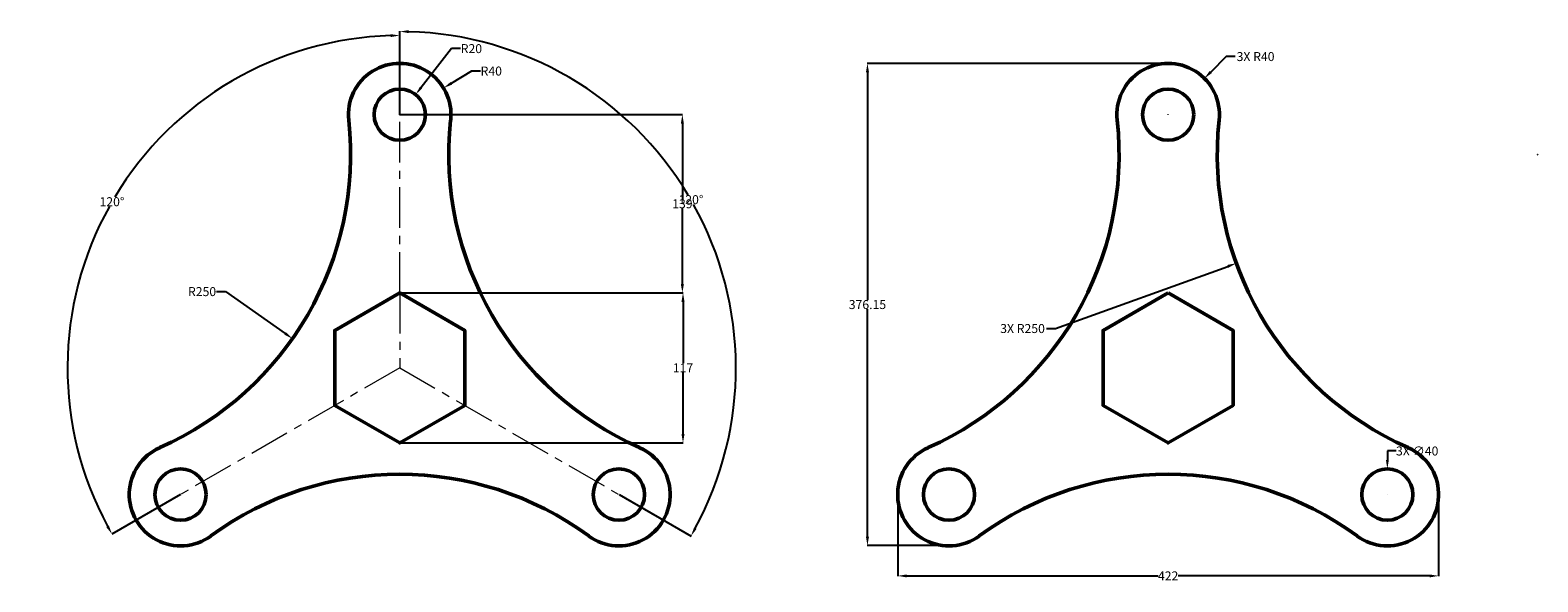
# Model space of a CAD drawing. Units: millimetres. Extents: x 13 to 1189, y 87 to 517.
import ezdxf

# ---------------------------------------------------------------- set-up
doc = ezdxf.new("R2010")
doc.units = ezdxf.units.MM
doc.header["$MEASUREMENT"] = 0
doc.linetypes.add('CENTER', pattern=[50.8, 31.75, -6.35, 6.35, -6.35])
for name, color, linetype, lineweight in [('M-CNTR', 7, 'CENTER', 18), ('M-DIMS', 3, 'Continuous', 25), ('M-OUTL', 7, 'Continuous', 50)]:
    doc.layers.add(name, color=color, linetype=linetype, lineweight=lineweight)
doc.styles.get("Standard").update_dxf_attribs({"font": 'arial.ttf'})
doc.dimstyles.get("Standard").update_dxf_attribs({"dimtxt": 7, "dimasz": 7, "dimexe": 0.18, "dimexo": 0.0625, "dimgap": 0.09, "dimtad": 0, "dimtih": 1, "dimtoh": 1, "dimdec": 1, "dimdsep": 46, "dimtxsty": 'Standard', "dimcen": 0.09, "dimadec": 0, "dimazin": 0, "dimtfac": 1, "dimtdec": 1, "dimtofl": 0, "dimtmove": 0, "dimatfit": 3, "dimfxl": 1, "dimtolj": 1, "dimtzin": 0, "dimarcsym": 0})

# ---------------------------------------------------------------- blocks, each defined once
blk = doc.blocks.new('*D1')
at = {"layer": 'Defpoints', "color": 0, "transparency": 16777216}
for p in [(301, 312.5), (522, 312.5), (301, 195.5)]:
    blk.add_point(p, dxfattribs=at)
at = {"layer": 'M-DIMS', "color": 0, "lineweight": -2, "transparency": 16777216}
for p, q in [((301.1, 312.5), (522.2, 312.5)), ((522, 305.5), (522, 257.6)), ((522, 202.5), (522, 250.4)), ((301.1, 195.5), (522.2, 195.5))]:
    blk.add_line(p, q, dxfattribs=at)
at = {"layer": 'M-DIMS', "color": 0, "transparency": 16777216}
for points in [[(520.8, 305.5), (523.2, 305.5), (522, 312.5)], [(520.8, 202.5), (523.2, 202.5), (522, 195.5)]]:
    blk.add_solid(points, dxfattribs=at)
at = {"layer": 'M-DIMS', "color": 0, "transparency": 16777216, "insert": (522, 254), "char_height": 7, "attachment_point": 5}
blk.add_mtext('\\A1;117', dxfattribs=at)
blk = doc.blocks.new('*D2')
at = {"layer": 'Defpoints', "color": 0, "transparency": 16777216}
for p in [(301, 451.5), (521.5, 451.5), (301, 312.5)]:
    blk.add_point(p, dxfattribs=at)
at = {"layer": 'M-DIMS', "color": 0, "lineweight": -2, "transparency": 16777216}
for p, q in [((301.1, 451.5), (521.7, 451.5)), ((521.5, 444.5), (521.5, 385.7)), ((521.5, 319.5), (521.5, 378.3)), ((301.1, 312.5), (521.7, 312.5))]:
    blk.add_line(p, q, dxfattribs=at)
at = {"layer": 'M-DIMS', "color": 0, "transparency": 16777216}
for points in [[(520.3, 444.5), (522.7, 444.5), (521.5, 451.5)], [(520.3, 319.5), (522.7, 319.5), (521.5, 312.5)]]:
    blk.add_solid(points, dxfattribs=at)
at = {"layer": 'M-DIMS', "color": 0, "transparency": 16777216, "insert": (521.5, 382), "char_height": 7, "attachment_point": 5}
blk.add_mtext('\\A1;139', dxfattribs=at)
blk = doc.blocks.new('*D3')
at = {"layer": 'Defpoints', "color": 0, "transparency": 16777216}
for p in [(313.4, 467.2), (301, 451.5)]:
    blk.add_point(p, dxfattribs=at)
at = {"layer": 'M-DIMS', "color": 0, "lineweight": -2, "transparency": 16777216}
for p, q in [((341.5, 503), (317.7, 472.7)), ((348.5, 503), (341.5, 503)), ((300.9, 451.5), (301.1, 451.5)), ((301, 451.4), (301, 451.6))]:
    blk.add_line(p, q, dxfattribs=at)
at = {"layer": 'M-DIMS', "color": 0, "transparency": 16777216}
blk.add_solid([(316.8, 473.4), (318.6, 472), (313.4, 467.2)], dxfattribs=at)
at = {"layer": 'M-DIMS', "color": 0, "transparency": 16777216, "insert": (356.9, 503), "char_height": 7, "attachment_point": 5}
blk.add_mtext('\\A1;R20', dxfattribs=at)
blk = doc.blocks.new('*D4')
at = {"layer": 'Defpoints', "color": 0, "transparency": 16777216}
for p in [(335.2, 472.3), (301, 451.5)]:
    blk.add_point(p, dxfattribs=at)
at = {"layer": 'M-DIMS', "color": 0, "lineweight": -2, "transparency": 16777216}
for p, q in [((357, 485.5), (341.2, 475.9)), ((364, 485.5), (357, 485.5)), ((300.9, 451.5), (301.1, 451.5)), ((301, 451.4), (301, 451.6))]:
    blk.add_line(p, q, dxfattribs=at)
at = {"layer": 'M-DIMS', "color": 0, "transparency": 16777216}
blk.add_solid([(340.6, 476.9), (341.8, 474.9), (335.2, 472.3)], dxfattribs=at)
at = {"layer": 'M-DIMS', "color": 0, "transparency": 16777216, "insert": (372.4, 485.5), "char_height": 7, "attachment_point": 5}
blk.add_mtext('\\A1;R40', dxfattribs=at)
blk = doc.blocks.new('*D5')
at = {"layer": 'Defpoints', "color": 0, "transparency": 16777216}
for p in [(12.7, 420.5), (217.3, 276.8)]:
    blk.add_point(p, dxfattribs=at)
at = {"layer": 'M-DIMS', "color": 0, "lineweight": -2, "transparency": 16777216}
for p, q in [((158, 313.5), (165, 313.5)), ((165, 313.5), (211.5, 280.8))]:
    blk.add_line(p, q, dxfattribs=at)
at = {"layer": 'M-DIMS', "color": 0, "transparency": 16777216}
blk.add_solid([(212.2, 281.8), (210.9, 279.9), (217.3, 276.8)], dxfattribs=at)
at = {"layer": 'M-DIMS', "color": 0, "transparency": 16777216, "insert": (146.8, 313.5), "char_height": 7, "attachment_point": 5}
blk.add_mtext('\\A1;R250', dxfattribs=at)
blk = doc.blocks.new('*D6')
at = {"layer": 'Defpoints', "color": 0, "transparency": 16777216}
for p in [(134.4, 452.6), (301, 451.5), (301, 312.5), (301, 254), (130, 155.2)]:
    blk.add_point(p, dxfattribs=at)
at = {"layer": 'M-DIMS', "color": 0, "lineweight": -2, "transparency": 16777216}
for p, q in [((301, 451.6), (301, 513.4)), ((129.9, 155.2), (76.3, 124.3))]:
    blk.add_line(p, q, dxfattribs=at)
for start, end in [(91.5471, 149.0605), (150.9307, 208.4529)]:
    blk.add_arc((301, 254), 259.2, start, end, dxfattribs=at)
at = {"layer": 'M-DIMS', "color": 0, "transparency": 16777216}
for points in [[(294, 514.3), (294, 512), (301, 513.2)], [(74.1, 131.1), (72, 129.9), (76.5, 124.4)]]:
    blk.add_solid(points, dxfattribs=at)
at = {"layer": 'M-DIMS', "color": 0, "transparency": 16777216, "insert": (76.5, 383.6), "char_height": 7, "attachment_point": 5}
blk.add_mtext('\\A1;120°', dxfattribs=at)
blk = doc.blocks.new('*D7')
at = {"layer": 'Defpoints', "color": 0, "transparency": 16777216}
for p in [(301, 451.5), (301, 312.5), (559.3, 299.6), (301, 254), (472, 155.2)]:
    blk.add_point(p, dxfattribs=at)
at = {"layer": 'M-DIMS', "color": 0, "lineweight": -2, "transparency": 16777216}
for p, q in [((301, 451.6), (301, 516.5)), ((472.1, 155.2), (528.3, 122.8))]:
    blk.add_line(p, q, dxfattribs=at)
for start, end in [(30.9285, 88.471), (331.529, 29.0801)]:
    blk.add_arc((301, 254), 262.3, start, end, dxfattribs=at)
at = {"layer": 'M-DIMS', "color": 0, "transparency": 16777216}
for points in [[(308, 515.1), (308, 517.4), (301, 516.3)], [(532.6, 128.4), (530.6, 129.5), (528.2, 122.8)]]:
    blk.add_solid(points, dxfattribs=at)
at = {"layer": 'M-DIMS', "color": 0, "transparency": 16777216, "insert": (528.2, 385.2), "char_height": 7, "attachment_point": 5}
blk.add_mtext('\\A1;120°', dxfattribs=at)
blk = doc.blocks.new('PLATE-3ARM-HEX')
blk.add_lwpolyline([(0, 58.5), (-50.7, 29.2), (-50.7, -29.3), (0, -58.5), (50.7, -29.3), (50.7, 29.2)], close=True)
for centre in [(0, 197.5), (-171, -98.8), (171, -98.8)]:
    blk.add_circle(centre, 20)
for centre, radius, start, end in [((0, 197.5), 40, 353.8577, 186.1423), ((-288.3, 166.5), 250, 293.8577, 6.1423), ((288.3, 166.5), 250, 173.8577, 246.1423), ((-171, -98.8), 40, 113.8577, 306.1423), ((171, -98.8), 40, 233.8577, 66.1423), ((0, -332.9), 250, 53.8577, 126.1423)]:
    blk.add_arc(centre, radius, start, end)
blk = doc.blocks.new('*D9')
at = {"layer": 'Defpoints', "color": 0, "transparency": 16777216}
for p in [(689.5, 156.7), (1111.5, 156.7), (1111.5, 91.8)]:
    blk.add_point(p, dxfattribs=at)
at = {"layer": 'M-DIMS', "color": 0, "lineweight": -2, "transparency": 16777216}
for p, q in [((689.5, 156.6), (689.5, 91.6)), ((1111.5, 156.6), (1111.5, 91.6)), ((696.5, 91.8), (892.6, 91.8)), ((1104.5, 91.8), (908.4, 91.8))]:
    blk.add_line(p, q, dxfattribs=at)
at = {"layer": 'M-DIMS', "color": 0, "transparency": 16777216}
for points in [[(696.5, 92.9), (696.5, 90.6), (689.5, 91.8)], [(1104.5, 92.9), (1104.5, 90.6), (1111.5, 91.8)]]:
    blk.add_solid(points, dxfattribs=at)
at = {"layer": 'M-DIMS', "color": 0, "transparency": 16777216, "insert": (900.5, 91.8), "char_height": 7, "attachment_point": 5}
blk.add_mtext('\\A1;422', dxfattribs=at)
blk = doc.blocks.new('*D10')
at = {"layer": 'Defpoints', "color": 0, "transparency": 16777216}
for p in [(665.9, 491.5), (900.5, 491.5), (732.3, 115.4)]:
    blk.add_point(p, dxfattribs=at)
at = {"layer": 'M-DIMS', "color": 0, "lineweight": -2, "transparency": 16777216}
for p, q in [((900.4, 491.5), (665.7, 491.5)), ((665.9, 484.5), (665.9, 307.1)), ((665.9, 122.4), (665.9, 299.8)), ((732.3, 115.4), (665.7, 115.4))]:
    blk.add_line(p, q, dxfattribs=at)
at = {"layer": 'M-DIMS', "color": 0, "transparency": 16777216}
for points in [[(664.7, 484.5), (667.1, 484.5), (665.9, 491.5)], [(664.7, 122.4), (667.1, 122.4), (665.9, 115.4)]]:
    blk.add_solid(points, dxfattribs=at)
at = {"layer": 'M-DIMS', "color": 0, "transparency": 16777216, "insert": (665.9, 303.4), "char_height": 7, "attachment_point": 5}
blk.add_mtext('\\A1;376.15', dxfattribs=at)
blk = doc.blocks.new('*D11')
at = {"layer": 'Defpoints', "color": 0, "transparency": 16777216}
for p in [(1071.5, 175.3), (1071.5, 135.3)]:
    blk.add_point(p, dxfattribs=at)
at = {"layer": 'M-DIMS', "color": 0, "lineweight": -2, "transparency": 16777216}
for p, q in [((1078.5, 189.2), (1071.5, 189.2)), ((1071.5, 189.2), (1071.5, 182.3)), ((1071.5, 155.3), (1071.6, 155.3)), ((1071.5, 155.2), (1071.5, 155.3))]:
    blk.add_line(p, q, dxfattribs=at)
at = {"layer": 'M-DIMS', "color": 0, "transparency": 16777216}
blk.add_solid([(1070.4, 182.3), (1072.7, 182.3), (1071.5, 175.3)], dxfattribs=at)
at = {"layer": 'M-DIMS', "color": 0, "transparency": 16777216, "insert": (1094.8, 189.2), "char_height": 7, "attachment_point": 5}
blk.add_mtext('\\A1;3X ∅40', dxfattribs=at)
blk = doc.blocks.new('*D12')
at = {"layer": 'Defpoints', "color": 0, "transparency": 16777216}
for p in [(928.8, 479.8), (900.5, 451.5)]:
    blk.add_point(p, dxfattribs=at)
at = {"layer": 'M-DIMS', "color": 0, "lineweight": -2, "transparency": 16777216}
for p, q in [((945.8, 496.8), (933.7, 484.7)), ((952.8, 496.8), (945.8, 496.8)), ((900.4, 451.5), (900.6, 451.5)), ((900.5, 451.4), (900.5, 451.6))]:
    blk.add_line(p, q, dxfattribs=at)
at = {"layer": 'M-DIMS', "color": 0, "transparency": 16777216}
blk.add_solid([(932.9, 485.6), (934.6, 483.9), (928.8, 479.8)], dxfattribs=at)
at = {"layer": 'M-DIMS', "color": 0, "transparency": 16777216, "insert": (968.7, 496.8), "char_height": 7, "attachment_point": 5}
blk.add_mtext('\\A1;3X R40', dxfattribs=at)
blk = doc.blocks.new('*D13')
at = {"layer": 'Defpoints', "color": 0, "transparency": 16777216}
for p in [(1188.8, 420.5), (953.7, 335.6)]:
    blk.add_point(p, dxfattribs=at)
at = {"layer": 'M-DIMS', "color": 0, "lineweight": -2, "transparency": 16777216}
for p, q in [((1188.7, 420.5), (1188.9, 420.5)), ((1188.8, 420.4), (1188.8, 420.6)), ((812.6, 284.7), (947.1, 333.2)), ((805.6, 284.7), (812.6, 284.7))]:
    blk.add_line(p, q, dxfattribs=at)
at = {"layer": 'M-DIMS', "color": 0, "transparency": 16777216}
blk.add_solid([(946.7, 334.3), (947.5, 332.1), (953.7, 335.6)], dxfattribs=at)
at = {"layer": 'M-DIMS', "color": 0, "transparency": 16777216, "insert": (786.9, 284.7), "char_height": 7, "attachment_point": 5}
blk.add_mtext('\\A1;3X R250', dxfattribs=at)

msp = doc.modelspace()

# ---------------------------------------------------------------- linework, layer by layer
at = {"layer": 'M-CNTR'}
for p, q in [((301, 312.5), (301, 451.5)), ((301, 312.5), (301, 254)), ((301, 254), (129.96, 155.25)), ((301, 254), (472.04, 155.25))]:
    msp.add_line(p, q, dxfattribs=at)

# ---------------------------------------------------------------- block references
at = {"layer": 'M-OUTL'}
for p in [(301, 254), (900.5, 254)]:
    msp.add_blockref('PLATE-3ARM-HEX', p, dxfattribs=at)

# ---------------------------------------------------------------- dimensions: what is measured, and where the dimension line sits
at = {"layer": 'M-DIMS', "transparency": 33554610}
for base, line1, line2, picture, middle in [((134.358, 452.597), ((301, 312.5), (301, 451.5)), ((301, 254), (129.96, 155.25)), '*D6', (76.483, 383.625)), ((559.329, 299.55), ((301, 254), (472.04, 155.25)), ((301, 312.5), (301, 451.5)), '*D7', (528.17, 385.157))]:
    dim = msp.add_angular_dim_2l(base=base, line1=line1, line2=line2, dimstyle='Standard', override={"dimclrd": 0, "dimclre": 0, "dimclrt": 0}, dxfattribs=at)
    dim.commit()
    dim.dimension.update_dxf_attribs({"geometry": picture, "text_midpoint": middle})
for center, mpoint, picture, middle in [((301, 451.5), (313.363, 467.221), '*D3', (356.941, 503)), ((301, 451.5), (335.192, 472.259), '*D4', (372.441, 485.5)), ((12.665, 420.47), (217.261, 276.802), '*D5', (146.839, 313.5))]:
    dim = msp.add_radius_dim(center=center, mpoint=mpoint, dimstyle='Standard', override={"dimclrd": 0, "dimclre": 0, "dimclrt": 0}, dxfattribs=at)
    dim.commit()
    dim.dimension.update_dxf_attribs({"geometry": picture, "text_midpoint": middle, "dimtype": 164})
at = {"layer": 'M-DIMS'}
for center, mpoint, picture, middle in [((900.5, 451.5), (928.784, 479.784), '*D12', (968.714, 496.755)), ((1188.835, 420.47), (953.684, 335.594), '*D13', (786.915, 284.669))]:
    dim = msp.add_radius_dim(center=center, mpoint=mpoint, text='3X <>', dimstyle='Standard', override={"dimdec": 0, "dimlfac": 1, "dimrnd": 0, "dimzin": 0, "dimdsep": 46, "dimlunit": 2}, dxfattribs=at)
    dim.commit()
    dim.dimension.update_dxf_attribs({"geometry": picture, "text_midpoint": middle, "dimtype": 164})
dim = msp.add_linear_dim(base=(665.886, 491.5), p1=(732.316, 115.352), p2=(900.5, 491.5), angle=90, dimstyle='Standard', override={"dimdec": 2, "dimlfac": 1, "dimrnd": 0, "dimzin": 0, "dimdsep": 46, "dimlunit": 2}, dxfattribs=at)
dim.commit()
dim.dimension.update_dxf_attribs({"geometry": '*D10', "text_midpoint": (665.886, 303.426)})
at = {"layer": 'M-DIMS', "transparency": 33554610}
for base, p1, p2, picture, middle in [((521.5, 451.5), (301, 312.5), (301, 451.5), '*D2', (521.5, 382)), ((522, 312.5), (301, 195.5), (301, 312.5), '*D1', (522, 254))]:
    dim = msp.add_linear_dim(base=base, p1=p1, p2=p2, angle=90, dimstyle='Standard', override={"dimclrd": 0, "dimclre": 0, "dimclrt": 0}, dxfattribs=at)
    dim.commit()
    dim.dimension.update_dxf_attribs({"geometry": picture, "text_midpoint": middle})
at = {"layer": 'M-DIMS'}
dim = msp.add_diameter_dim_2p(p1=(1071.54, 135.25), p2=(1071.54, 175.25), text='3X <>', dimstyle='Standard', override={"dimdec": 0, "dimlfac": 1, "dimrnd": 0, "dimzin": 0, "dimdsep": 46, "dimlunit": 2}, dxfattribs=at)
dim.commit()
dim.dimension.update_dxf_attribs({"geometry": '*D11', "text_midpoint": (1094.772, 189.25)})
dim = msp.add_linear_dim(base=(1111.514, 91.752), p1=(689.486, 156.679), p2=(1111.514, 156.679), dimstyle='Standard', override={"dimdec": 0, "dimlfac": 1, "dimrnd": 0, "dimzin": 0, "dimdsep": 46, "dimlunit": 2}, dxfattribs=at)
dim.commit()
dim.dimension.update_dxf_attribs({"geometry": '*D9', "text_midpoint": (900.5, 91.752)})

doc.saveas('drawing.dxf')
